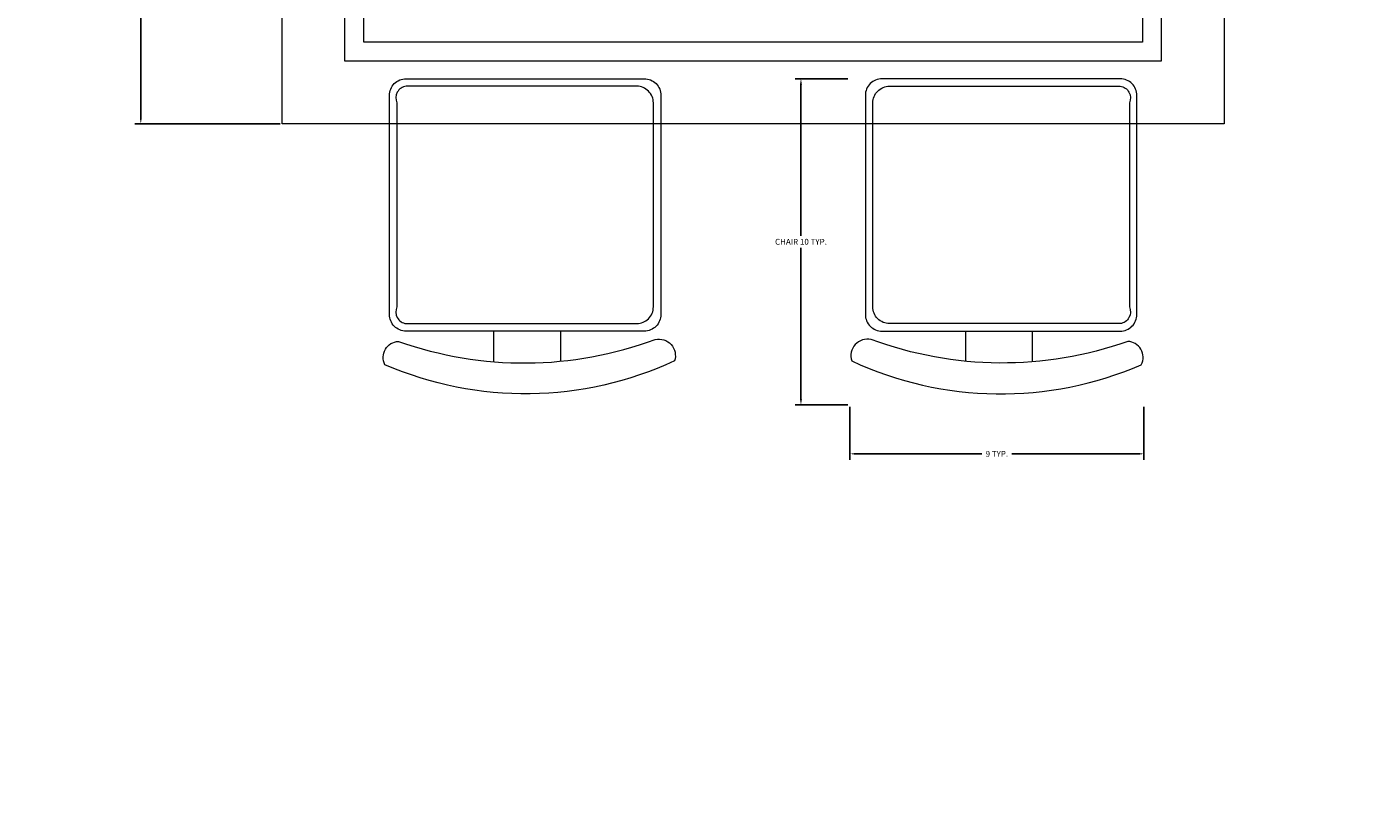
# Model space of a CAD drawing. Units: inches. Extents: x 1088 to 1703, y 668 to 1875.
# Tile 20 of 45: x 1371 to 1413, y 1623 to 1648. Entities that reach past the tile are written whole.
import ezdxf

# ---------------------------------------------------------------- set-up
doc = ezdxf.new("R2010")
doc.units = ezdxf.units.IN
doc.layers.add('A-ANNO-DIMS', color=2, linetype='Continuous', lineweight=18)
doc.layers.add('A-FURN', color=8, linetype='Continuous', lineweight=13)
doc.styles.get("Standard").update_dxf_attribs({"font": 'arial.ttf'})
doc.dimstyles.get("Standard").update_dxf_attribs({"dimtxt": 0.18, "dimasz": 0.18, "dimexe": 0.18, "dimexo": 0.0625, "dimgap": 0.09, "dimtad": 0, "dimtih": 1, "dimtoh": 1, "dimdec": 4, "dimzin": 0, "dimdsep": 46, "dimtxsty": 'Standard', "dimcen": 0.09, "dimadec": 0, "dimazin": 0, "dimtfac": 1, "dimtdec": 4, "dimtofl": 0, "dimtmove": 0, "dimatfit": 3, "dimfxl": 1, "dimtolj": 1, "dimtzin": 0, "dimarcsym": 0})

# ---------------------------------------------------------------- blocks, each defined once
blk = doc.blocks.new('TABLE-DINING-RECT')
for points in [[(0, 17.407), (29.011, 17.407), (29.011, 0), (0, 0)], [(1.934, 15.473), (27.077, 15.473), (27.077, 1.934), (1.934, 1.934)], [(2.514, 14.892), (26.497, 14.892), (26.497, 2.515), (2.514, 2.515)]]:
    blk.add_lwpolyline(points, close=True)
blk = doc.blocks.new('CHAIR-DINING')
for points in [[(7.771, 8.293, 0.414214), (7.258, 8.807), (0.513, 8.807, 0.414214), (0, 8.293), (0, 0.958, 0.414214), (0.513, 0.444), (7.258, 0.444, 0.414214), (7.771, 0.958), (7.771, 8.293)], [(8.088, 8.524, -0.175809), (8.029, 0.622, 0.578392), (8.687, 0.024, 0.214524), (8.806, 8.943, 0.552014), (8.088, 8.524, -0.065079)], [(7.771, 3.534), (8.699, 3.534, -0.064759)]]:
    blk.add_lwpolyline(points, format="xyb")
blk.add_lwpolyline([(7.54, 8.29), (7.54, 1.189, -0.414214), (7.027, 0.676), (0.744, 0.676, -0.414214), (0.231, 1.189), (0.231, 8.29, -0.512069), (0.744, 8.575), (7.027, 8.575, -0.512069)], format="xyb", close=True)
blk.add_lwpolyline([(8.716, 5.588), (7.771, 5.588)])
blk = doc.blocks.new('*D14')
at = {"layer": 'A-ANNO-DIMS', "color": 0, "lineweight": -2, "transparency": 16777216}
for p, q in [((1396.764, 1646.07), (1395.139, 1646.07)), ((1395.319, 1645.89), (1395.319, 1641.231)), ((1395.319, 1636.205), (1395.319, 1640.864)), ((1396.764, 1636.025), (1395.139, 1636.025))]:
    blk.add_line(p, q, dxfattribs=at)
at = {"layer": 'A-ANNO-DIMS', "color": 0, "transparency": 16777216}
for points in [[(1395.289, 1645.89), (1395.349, 1645.89), (1395.319, 1646.07)], [(1395.289, 1636.205), (1395.349, 1636.205), (1395.319, 1636.025)]]:
    blk.add_solid(points, dxfattribs=at)
at = {"layer": 'Defpoints', "color": 0, "transparency": 16777216}
for p in [(1396.826, 1646.07), (1395.319, 1636.025), (1396.826, 1636.025)]:
    blk.add_point(p, dxfattribs=at)
at = {"layer": 'A-ANNO-DIMS', "color": 0, "transparency": 16777216, "insert": (1395.319, 1641.048), "char_height": 0.18, "attachment_point": 5}
blk.add_mtext('\\A1;CHAIR 10 TYP.', dxfattribs=at)
blk = doc.blocks.new('*D15')
at = {"layer": 'A-ANNO-DIMS', "color": 0, "lineweight": -2, "transparency": 16777216}
for p, q in [((1396.826, 1635.963), (1396.826, 1634.339)), ((1405.88, 1635.963), (1405.88, 1634.339)), ((1397.006, 1634.519), (1400.895, 1634.519)), ((1405.7, 1634.519), (1401.811, 1634.519))]:
    blk.add_line(p, q, dxfattribs=at)
at = {"layer": 'A-ANNO-DIMS', "color": 0, "transparency": 16777216}
for points in [[(1397.006, 1634.549), (1397.006, 1634.489), (1396.826, 1634.519)], [(1405.7, 1634.549), (1405.7, 1634.489), (1405.88, 1634.519)]]:
    blk.add_solid(points, dxfattribs=at)
at = {"layer": 'Defpoints', "color": 0, "transparency": 16777216}
for p in [(1396.826, 1636.025), (1405.88, 1636.025), (1405.88, 1634.519)]:
    blk.add_point(p, dxfattribs=at)
at = {"layer": 'A-ANNO-DIMS', "color": 0, "transparency": 16777216, "insert": (1401.353, 1634.519), "char_height": 0.18, "attachment_point": 5}
blk.add_mtext('\\A1;9 TYP.', dxfattribs=at)
blk = doc.blocks.new('*D17')
at = {"layer": 'A-ANNO-DIMS', "color": 0, "lineweight": -2, "transparency": 16777216}
for p, q in [((1379.276, 1662.086), (1374.807, 1662.086)), ((1374.987, 1661.906), (1374.987, 1653.563)), ((1374.987, 1644.86), (1374.987, 1653.203)), ((1379.276, 1644.68), (1374.807, 1644.68))]:
    blk.add_line(p, q, dxfattribs=at)
at = {"layer": 'A-ANNO-DIMS', "color": 0, "transparency": 16777216}
for points in [[(1374.957, 1661.906), (1375.017, 1661.906), (1374.987, 1662.086)], [(1374.957, 1644.86), (1375.017, 1644.86), (1374.987, 1644.68)]]:
    blk.add_solid(points, dxfattribs=at)
at = {"layer": 'Defpoints', "color": 0, "transparency": 16777216}
for p in [(1374.987, 1662.086), (1379.339, 1662.086), (1379.339, 1644.68)]:
    blk.add_point(p, dxfattribs=at)
at = {"layer": 'A-ANNO-DIMS', "color": 0, "transparency": 16777216, "insert": (1374.987, 1653.383), "char_height": 0.18, "attachment_point": 5}
blk.add_mtext('\\A1;17 TYP.', dxfattribs=at)
blk = doc.blocks.new('*D38')
at = {"layer": 'A-ANNO-DIMS', "color": 0, "lineweight": -2, "transparency": 16777216}
for p, q in [((1317.345, 1736.945), (1317.345, 725.549)), ((1437.345, 1736.945), (1437.345, 725.549)), ((1317.525, 725.729), (1377.065, 725.729)), ((1437.165, 725.729), (1377.625, 725.729))]:
    blk.add_line(p, q, dxfattribs=at)
at = {"layer": 'A-ANNO-DIMS', "color": 0, "transparency": 16777216}
for points in [[(1317.525, 725.759), (1317.525, 725.699), (1317.345, 725.729)], [(1437.165, 725.759), (1437.165, 725.699), (1437.345, 725.729)]]:
    blk.add_solid(points, dxfattribs=at)
at = {"layer": 'Defpoints', "color": 0, "transparency": 16777216}
for p in [(1317.345, 1737.007), (1437.345, 1737.007), (1437.345, 725.729)]:
    blk.add_point(p, dxfattribs=at)
at = {"layer": 'A-ANNO-DIMS', "color": 0, "transparency": 16777216, "insert": (1377.345, 725.729), "char_height": 0.18, "attachment_point": 5}
blk.add_mtext('\\A1;120', dxfattribs=at)

msp = doc.modelspace()

# ---------------------------------------------------------------- linework, layer by layer
at = {"layer": 'A-FURN'}
for points in [[(1390.493, 1638.298), (1383.158, 1638.298, -0.414214), (1382.644, 1638.811), (1382.644, 1645.556, -0.414214), (1383.158, 1646.07), (1390.493, 1646.07, -0.414214), (1391.007, 1645.556), (1391.007, 1638.811, -0.414214), (1390.493, 1638.298)], [(1390.829, 1638.041, -0.578392), (1391.427, 1637.383, -0.214524), (1382.508, 1637.263, -0.552014), (1382.927, 1637.981, 0.175809), (1390.829, 1638.041)], [(1387.917, 1638.298), (1387.917, 1637.37, 0.064759)]]:
    msp.add_lwpolyline(points, format="xyb", dxfattribs=at)
msp.add_lwpolyline([(1383.161, 1638.529), (1390.262, 1638.529, 0.414214), (1390.775, 1639.043), (1390.775, 1645.325, 0.414214), (1390.262, 1645.838), (1383.161, 1645.838, 0.512069), (1382.876, 1645.325), (1382.876, 1639.043, 0.512069)], format="xyb", close=True, dxfattribs=at)
msp.add_lwpolyline([(1385.863, 1637.354), (1385.863, 1638.298)], dxfattribs=at)

# ---------------------------------------------------------------- block references
msp.add_blockref('TABLE-DINING-RECT', (1379.339, 1644.68), dxfattribs=at)
at = {"layer": 'A-FURN', "rotation": 270.0000011876089}
msp.add_blockref('CHAIR-DINING', (1396.858, 1646.069), dxfattribs=at)

# ---------------------------------------------------------------- dimensions: what is measured, and where the dimension line sits
at = {"layer": 'A-ANNO-DIMS'}
dim = msp.add_linear_dim(base=(1437.345, 725.729), p1=(1317.345, 1737.007), p2=(1437.345, 1737.007), dimstyle='Standard', override={"dimdec": 0, "dimlfac": 1, "dimrnd": 0, "dimzin": 0, "dimdsep": 46, "dimlunit": 2}, dxfattribs=at)
dim.commit()
dim.dimension.update_dxf_attribs({"geometry": '*D38', "text_midpoint": (1377.345, 725.729)})
for base, p1, p2, angle, text, picture, middle in [((1374.987, 1662.086), (1379.339, 1644.68), (1379.339, 1662.086), 90, '<> TYP.', '*D17', (1374.987, 1653.383)), ((1395.319, 1636.025), (1396.826, 1646.07), (1396.826, 1636.025), 270, 'CHAIR <> TYP.', '*D14', (1395.319, 1641.048)), ((1405.88, 1634.519), (1396.826, 1636.025), (1405.88, 1636.025), 0, '<> TYP.', '*D15', (1401.353, 1634.519))]:
    dim = msp.add_linear_dim(base=base, p1=p1, p2=p2, angle=angle, text=text, dimstyle='Standard', override={"dimdec": 0, "dimlfac": 1, "dimrnd": 0, "dimzin": 0, "dimdsep": 46, "dimlunit": 2}, dxfattribs=at)
    dim.commit()
    dim.dimension.update_dxf_attribs({"geometry": picture, "text_midpoint": middle})

doc.saveas('drawing.dxf')
